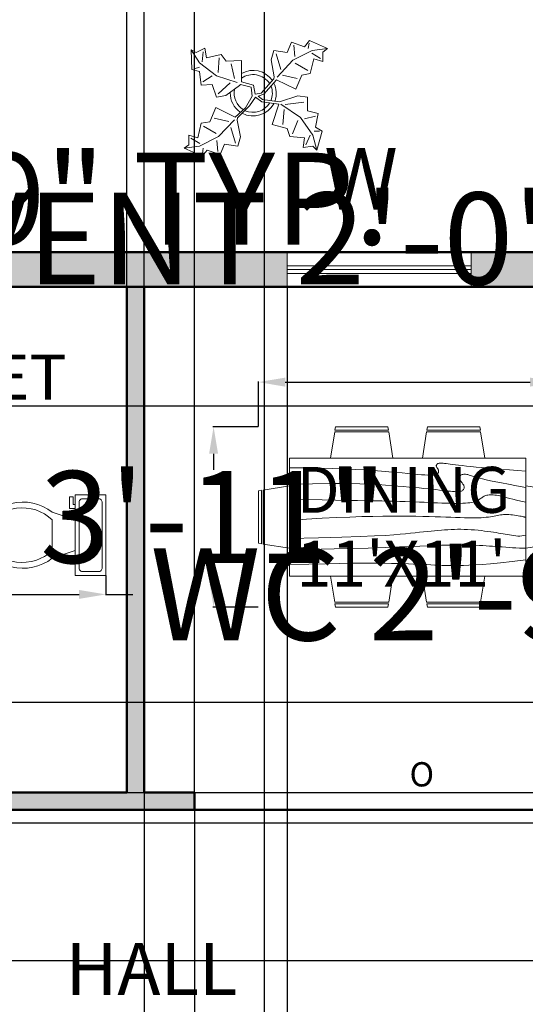
# Model space of a CAD drawing. Units: inches. Extents: x -166 to 1001, y 0 to 688.
# Tile 6 of 11: x 229 to 361, y 287 to 544. Entities that reach past the tile are written whole.
import ezdxf

# ---------------------------------------------------------------- set-up
doc = ezdxf.new("R2010")
doc.units = ezdxf.units.IN
doc.header["$MEASUREMENT"] = 0
for name, color, linetype, lineweight in [('A-ANNO-DIMS', 1, 'Continuous', 18), ('A-ANNO-TEXT', 2, 'Continuous', 25), ('A-AREA-IDEN', 2, 'Continuous', 25), ('A-FLOR-FIXT', 11, 'Continuous', 18), ('A-GLAZ', 130, 'Continuous', 18), ('A-WALL-PATT', 5, 'Continuous', 13), ('FURNITURE', 11, 'Continuous', 18), ('TREES', 80, 'Continuous', 13), ('WALLS', 250, 'Continuous', 50)]:
    doc.layers.add(name, color=color, linetype=linetype, lineweight=lineweight)
doc.styles.get("Standard").update_dxf_attribs({"font": 'arial.ttf'})
doc.dimstyles.get("Standard").update_dxf_attribs({"dimtxt": 24, "dimasz": 7, "dimexe": 0.18, "dimexo": 0.0625, "dimgap": 0.09, "dimtad": 0, "dimtih": 1, "dimtoh": 1, "dimdec": 0, "dimzin": 0, "dimdsep": 46, "dimlunit": 3, "dimtxsty": 'Standard', "dimcen": 0.09, "dimadec": 0, "dimazin": 0, "dimtfac": 1, "dimtdec": 0, "dimtofl": 0, "dimtmove": 0, "dimatfit": 3, "dimfxl": 1, "dimtolj": 1, "dimtzin": 0, "dimarcsym": 0})

# ---------------------------------------------------------------- blocks, each defined once
blk = doc.blocks.new('Toilet - top')
for p, q in [((9.5, -6), (9.5, -2)), ((-10, -8.5), (-8, -8.5)), ((-10, -9.5), (-10, -8.5)), ((-7, -9.5), (-10, -9.5)), ((-8, -8.5), (-8, -8)), ((-7, -8), (-7, -9.5)), ((-4, -8), (-6, -14)), ((4, -8), (6, -14)), ((4, -14), (-4, -14))]:
    blk.add_line(p, q)
blk.add_lwpolyline([(10.5, -8), (10.5, 0), (-10.5, 0), (-10.5, -8)], close=True)
for points in [[(-9.5, -2), (-9.5, -6)], [(8.5, -1), (-8.5, -1)], [(-8.5, -7), (8.5, -7)]]:
    blk.add_lwpolyline(points)
for centre, radius, start, end in [((-8.62, -1.88), 0.884, 81.8699, 188.1301), ((8.62, -1.88), 0.884, 351.8699, 98.1301), ((-8.62, -6.12), 0.884, 171.8699, 278.1301), ((8.62, -6.12), 0.884, 261.8699, 8.1301), ((3.52, -21.58), 12.17, 141.4691, 247.9714), ((4.2, -21.82), 11.33, 136.3677, 238.9468), ((-3.52, -21.58), 12.17, 292.0284, 38.5307), ((-4.2, -21.82), 11.33, 301.053, 43.6321), ((0, -27.88), 4, 245.7318, 294.2682), ((0, -29), 4, 254.8605, 285.1395)]:
    blk.add_arc(centre, radius, start, end)
blk = doc.blocks.new('Dining Set - 36 x 72 in.')
for p, q in [((-22, 27.5), (-22.1562, 26.50042)), ((-22, 27.5), (-6, 27.5)), ((-5.8437, 26.49966), (-6, 27.5)), ((6, 27.5), (5.8438, 26.50042)), ((6, 27.5), (22, 27.5)), ((22.1563, 26.49966), (22, 27.5)), ((-22.2343, 26.00059), (-23.4847, 17.99762)), ((-22.2304, 26), (-5.7608, 26)), ((-5.8416, 26.5), (-22.1534, 26.5)), ((-4.5152, 17.99762), (-5.7655, 25.99926)), ((5.7657, 26.00059), (4.5153, 17.99762)), ((5.7696, 26), (22.2392, 26)), ((22.1584, 26.5), (5.8466, 26.5)), ((23.4848, 17.99762), (22.2345, 25.99926)), ((36, 18), (-36, 18)), ((-36, 18), (-36, -18)), ((36, -18), (36, 18)), ((-44.0006, 8.23428), (-35.9976, 9.48474)), ((44.0006, 8.23428), (35.9976, 9.48474)), ((-45.5, 8), (-44.5004, 8.15617)), ((-45.5, 8), (-45.5, -8)), ((-44.5, -8.15843), (-44.5, 8.15338)), ((-44, 8.23041), (-44, -8.23915)), ((44, 8.23041), (44, -8.23915)), ((44.5, -8.15843), (44.5, 8.15338)), ((45.5, 8), (44.5005, 8.15617)), ((45.5, 8), (45.5, -8)), ((-44.4997, -8.15631), (-45.5, -8)), ((-35.9976, -9.48476), (-43.9993, -8.2345)), ((35.9976, -9.48476), (43.9993, -8.2345)), ((44.4997, -8.15631), (45.5, -8)), ((-36, -18), (36, -18)), ((-22.2343, -26.0006), (-23.4847, -17.99762)), ((-4.5152, -17.99762), (-5.7655, -25.99928)), ((5.7657, -26.0006), (4.5153, -17.99762)), ((23.4848, -17.99762), (22.2345, -25.99928)), ((-22.2304, -26), (-5.7608, -26)), ((-22, -27.5), (-22.1562, -26.50044)), ((-5.8416, -26.5), (-22.1534, -26.5)), ((-5.8437, -26.49967), (-6, -27.5)), ((5.7696, -26), (22.2392, -26)), ((6, -27.5), (5.8438, -26.50044)), ((22.1584, -26.5), (5.8466, -26.5)), ((22.1563, -26.49967), (22, -27.5)), ((-22, -27.5), (-6, -27.5)), ((6, -27.5), (22, -27.5))]:
    blk.add_line(p, q)
for points in [[(-36, 15), (-31.1772, 14.97754), (-26.8079, 14.91406), (-22.8538, 14.81543), (-19.276, 14.6875), (-16.0362, 14.53613), (-13.0957, 14.36718), (-10.4159, 14.18652), (-7.9583, 14), (-5.6904, 13.81315), (-3.6035, 13.63021), (-1.6954, 13.45508), (0.0365, 13.29166), (1.5945, 13.14388), (2.9811, 13.01562), (4.1988, 12.9108), (5.25, 12.83333), (6.1393, 12.78613), (6.8802, 12.76823), (7.4883, 12.77767), (7.9792, 12.8125), (8.3685, 12.87077), (8.6719, 12.95052), (8.9049, 13.0498), (9.0833, 13.16666), (9.2205, 13.29899), (9.3216, 13.44401), (9.3895, 13.59879), (9.4271, 13.76041), (9.4373, 13.92594), (9.4232, 14.09245), (9.3875, 14.257), (9.3333, 14.41666), (9.2638, 14.56917), (9.1836, 14.71484), (9.0975, 14.85465), (9.0104, 14.98958), (8.9272, 15.1206), (8.8529, 15.2487), (8.7922, 15.37483), (8.75, 15.5), (8.7305, 15.62467), (8.7344, 15.74739), (8.7617, 15.86621), (8.8125, 15.97916), (8.8867, 16.08431), (8.9844, 16.17968), (9.1055, 16.26334), (9.25, 16.33333), (9.4189, 16.38802), (9.6172, 16.42708), (9.8506, 16.45052), (10.125, 16.45833), (10.4463, 16.45052), (10.8203, 16.42708), (11.2529, 16.38802), (11.75, 16.33333), (12.3184, 16.26318), (12.9694, 16.17838), (13.7151, 16.07991), (14.5677, 15.96875), (15.5395, 15.84586), (16.6426, 15.71224), (17.8893, 15.56884), (19.2917, 15.41666), (20.859, 15.25667), (22.5879, 15.08984), (24.4721, 14.91715), (26.5052, 14.73958), (28.6809, 14.5581), (30.9929, 14.3737), (33.4347, 14.18733), (36, 14)], [(-36, 10), (-28.9766, 10.14274), (-23.1725, 10.20442), (-18.4241, 10.19775), (-14.5677, 10.13541), (-11.4399, 10.03011), (-8.877, 9.89453), (-6.7154, 9.74137), (-4.7917, 9.58333), (-2.9698, 9.43082), (-1.2246, 9.28515), (0.4415, 9.14534), (2.026, 9.01041), (3.5266, 8.87939), (4.9408, 8.7513), (6.266, 8.62516), (7.5, 8.5), (8.6411, 8.37549), (9.6914, 8.2539), (10.6538, 8.13818), (11.5312, 8.03125), (12.3267, 7.93603), (13.043, 7.85547), (13.6831, 7.79248), (14.25, 7.75), (14.7471, 7.7303), (15.1797, 7.73307), (15.5537, 7.75732), (15.875, 7.80208), (16.1494, 7.86637), (16.3828, 7.94922), (16.5811, 8.04964), (16.75, 8.16666), (16.8944, 8.29915), (17.0143, 8.44531), (17.1089, 8.60319), (17.1771, 8.77083), (17.218, 8.94629), (17.2305, 9.1276), (17.2137, 9.31282), (17.1667, 9.5), (17.0895, 9.6875), (16.987, 9.875), (16.8649, 10.0625), (16.7292, 10.25), (16.5856, 10.4375), (16.4401, 10.625), (16.2985, 10.8125), (16.1667, 11), (16.05, 11.18733), (15.9518, 11.3737), (15.8752, 11.5581), (15.8229, 11.73958), (15.798, 11.91715), (15.8034, 12.08984), (15.842, 12.25667), (15.9167, 12.41666), (16.0295, 12.56836), (16.1784, 12.70833), (16.3605, 12.83268), (16.5729, 12.9375), (16.8127, 13.01888), (17.0768, 13.07291), (17.3625, 13.0957), (17.6667, 13.08333), (17.9894, 13.03312), (18.3418, 12.94726), (18.7382, 12.82918), (19.1927, 12.68229), (19.7195, 12.51001), (20.3327, 12.31575), (21.0465, 12.10294), (21.875, 11.875), (22.8357, 11.63354), (23.959, 11.37304), (25.2786, 11.08618), (26.8282, 10.76562), (28.6414, 10.40405), (30.752, 9.99414), (33.1936, 9.52856), (36, 9)], [(-36, 5.5), (-30.7157, 5.3348), (-26.069, 5.20963), (-21.9946, 5.11767), (-18.4271, 5.05208), (-15.3009, 5.00602), (-12.5508, 4.97265), (-10.1112, 4.94515), (-7.9167, 4.91666), (-5.909, 4.88167), (-4.0586, 4.83984), (-2.3429, 4.79215), (-0.7396, 4.73958), (0.7739, 4.6831), (2.22, 4.6237), (3.6213, 4.56233), (5, 4.5), (6.373, 4.43782), (7.7344, 4.3776), (9.0723, 4.32129), (10.375, 4.27083), (11.6309, 4.22819), (12.8281, 4.19531), (13.9551, 4.17415), (15, 4.16666), (15.954, 4.17448), (16.819, 4.19791), (17.6001, 4.23698), (18.3021, 4.29166), (18.9299, 4.36198), (19.4883, 4.44791), (19.9823, 4.54948), (20.4167, 4.66666), (20.7969, 4.79899), (21.1302, 4.94401), (21.4245, 5.09879), (21.6875, 5.26041), (21.9271, 5.42594), (22.1511, 5.59245), (22.3672, 5.757), (22.5834, 5.91666), (22.8065, 6.06868), (23.0404, 6.21093), (23.2879, 6.34147), (23.5521, 6.45833), (23.8358, 6.55957), (24.142, 6.64323), (24.4735, 6.70735), (24.8334, 6.75), (25.2235, 6.76969), (25.642, 6.76692), (26.0858, 6.74267), (26.5521, 6.69791), (27.0379, 6.63362), (27.5404, 6.55078), (28.0565, 6.45036), (28.5834, 6.33333), (29.1242, 6.19987), (29.7071, 6.04687), (30.3661, 5.87044), (31.1354, 5.66666), (32.0493, 5.43164), (33.142, 5.16146), (34.4475, 4.85221), (36, 4.5)], [(-36, -1), (-30.7915, -0.6591), (-26.0195, -0.38216), (-21.6519, -0.16284), (-17.6563, 0.00521), (-14.0005, 0.12833), (-10.6523, 0.21289), (-7.5796, 0.26522), (-4.75, 0.29166), (-2.134, 0.29793), (0.2878, 0.28711), (2.5317, 0.26163), (4.6146, 0.22396), (6.5529, 0.17651), (8.3633, 0.12174), (10.0623, 0.06209), (11.6667, 0), (13.1899, -0.06201), (14.6341, -0.1211), (15.9982, -0.17432), (17.2813, -0.21875), (18.4823, -0.25147), (19.6003, -0.26953), (20.6343, -0.27002), (21.5834, -0.25), (22.4481, -0.20768), (23.2357, -0.14584), (23.9549, -0.06836), (24.6146, 0.02083), (25.2235, 0.11784), (25.7904, 0.21875), (26.3241, 0.31966), (26.8334, 0.41666), (27.3265, 0.50618), (27.8099, 0.58593), (28.2894, 0.65397), (28.7709, 0.70833), (29.2601, 0.74707), (29.763, 0.76823), (30.2855, 0.76985), (30.8334, 0.75), (31.4088, 0.70784), (31.9994, 0.64713), (32.589, 0.57275), (33.1615, 0.48958), (33.7008, 0.4025), (34.1908, 0.3164), (34.6153, 0.23616), (34.9584, 0.16666), (35.2099, 0.11165), (35.3848, 0.07031), (35.504, 0.04069), (35.5886, 0.02083), (35.6594, 0.00879), (35.7377, 0.0026), (35.8442, 0.00032), (36, 0)], [(-36, -6.5), (-27.1843, -6.31267), (-20.084, -6.1263), (-14.469, -5.9419), (-10.1094, -5.76042), (-6.7752, -5.58285), (-4.2363, -5.41016), (-2.2629, -5.24333), (-0.625, -5.08334), (0.8708, -4.93099), (2.2715, -4.78646), (3.5872, -4.64974), (4.8281, -4.52084), (6.0046, -4.39974), (7.127, -4.28646), (8.2053, -4.18099), (9.25, -4.08334), (10.2705, -3.99382), (11.2734, -3.91407), (12.2647, -3.84603), (13.25, -3.79167), (14.2354, -3.75293), (15.2266, -3.73177), (16.2295, -3.73015), (17.25, -3.75), (18.2912, -3.79248), (19.3451, -3.85547), (20.4009, -3.93604), (21.4479, -4.03125), (22.4754, -4.13819), (23.4727, -4.25391), (24.4289, -4.37549), (25.3334, -4.5), (26.1785, -4.62492), (26.9694, -4.74935), (27.7145, -4.87281), (28.4219, -4.99479), (29.1, -5.11483), (29.7572, -5.23242), (30.4016, -5.34709), (31.0417, -5.45834), (31.6837, -5.56437), (32.3262, -5.65821), (32.9658, -5.73153), (33.599, -5.77604), (34.2224, -5.78345), (34.8327, -5.74545), (35.4264, -5.65373), (36, -5.5)], [(-36, -10), (-26.4022, -9.81299), (-18.4675, -9.62891), (-11.9839, -9.45069), (-6.7396, -9.28125), (-2.5226, -9.12354), (0.8789, -8.98047), (3.6769, -8.85498), (6.0833, -8.75), (8.2767, -8.66765), (10.3021, -8.60677), (12.1712, -8.56543), (13.8958, -8.54167), (15.4876, -8.53353), (16.9583, -8.53907), (18.3197, -8.55632), (19.5834, -8.58334), (20.7616, -8.61841), (21.8685, -8.66081), (22.9188, -8.71004), (23.9271, -8.76563), (24.9081, -8.82707), (25.8763, -8.89388), (26.8465, -8.96558), (27.8334, -9.04167), (28.8474, -9.12118), (29.8828, -9.20117), (30.93, -9.27824), (31.9792, -9.34896), (33.0205, -9.40991), (34.0443, -9.45768), (35.0407, -9.48885), (36, -9.5)], [(-36, -14.5), (-30.0881, -14.33513), (-25.0332, -14.21224), (-20.7312, -14.12647), (-17.0781, -14.07292), (-13.97, -14.04671), (-11.3027, -14.04297), (-8.9724, -14.05681), (-6.875, -14.08334), (-4.9224, -14.11833), (-3.0905, -14.16016), (-1.3709, -14.20785), (0.2448, -14.26042), (1.7647, -14.3169), (3.1973, -14.3763), (4.5507, -14.43767), (5.8333, -14.5), (7.0554, -14.5621), (8.235, -14.62175), (9.3922, -14.67652), (10.5469, -14.72396), (11.7192, -14.76164), (12.929, -14.78711), (14.1965, -14.79794), (15.5417, -14.79167), (16.9933, -14.76424), (18.6152, -14.70508), (20.4804, -14.60197), (22.6615, -14.44271), (25.2312, -14.21509), (28.2624, -13.9069), (31.8277, -13.50594), (36, -13)]]:
    blk.add_lwpolyline(points)
blk = doc.blocks.new('Plant - Rubber or Philodendron')
for p, q in [((8.8871, 10.7908), (9.9809, 13.4933)), ((9.9809, 13.4933), (13.3837, 12.301)), ((13.3837, 12.301), (14.68, 13.9039)), ((14.5816, 13.2037), (14.3848, 11.8033)), ((14.68, 13.9039), (19.3848, 11.8146)), ((-16.2005, 11.4774), (-13.9899, 8.1064)), ((-16.2005, 11.4774), (-14.8639, 10.7964)), ((-16.0159, 6.3329), (-16.2005, 11.4774)), ((-14.8639, 10.7964), (-12.6195, 11.8975)), ((-13.3174, 8.325), (-13.0735, 11.0065)), ((-12.6195, 11.8975), (-12.1909, 9.4345)), ((-12.1909, 9.4345), (-8.3829, 10.3)), ((-8.3829, 10.3), (-7.0549, 8.501)), ((4.6914, 8.8812), (5.3859, 11.2828)), ((5.3859, 11.2828), (8.8871, 10.7908)), ((5.9878, 10.4842), (7.1971, 6.3869)), ((15.3859, 11.3055), (10.3916, 8.7942)), ((10.5828, 12.6946), (10.8893, 9.7953)), ((15.2875, 10.6053), (17.5907, 9.2105)), ((19.3848, 11.8146), (15.3859, 11.3055)), ((19.3848, 11.8146), (18.1868, 10.9119)), ((18.1868, 10.9119), (18.1925, 8.4119)), ((-13.9899, 8.1064), (-9.5434, 4.7185)), ((-8.8369, 9.409), (-9.0894, 5.6095)), ((-7.0549, 8.501), (-3.0284, 8.6941)), ((-4.8529, 4.012), (-5.7184, 7.82)), ((-3.0284, 8.6941), (-3.0709, 3.1041)), ((4.6914, 8.8812), (5.5014, 4.4831)), ((10.3916, 8.7942), (6.2847, 4.4028)), ((14.2977, 6.1031), (10.9934, 7.9956)), ((15.7909, 9.1065), (14.8995, 5.3044)), ((18.1925, 8.4119), (15.7909, 9.1065)), ((-14.0069, 5.8704), (-16.0159, 6.3329)), ((-15.3434, 6.5514), (-13.9984, 6.9884)), ((-13.5868, 2.2894), (-14.0069, 5.8704)), ((14.8995, 5.3044), (12.7005, 4.8994)), ((-13.1329, 3.1804), (-10.6614, 4.727)), ((-9.5434, 4.7185), (-4.1917, 2.9888)), ((-9.1318, 0.0195), (-5.9793, 2.9025)), ((-3.0709, 3.1041), (0.0797, 2.3163)), ((2.1141, 0.2298), (5.4346, 3.9146)), ((6.1032, 3.6844), (2.8262, -0.031)), ((5.4346, 3.9146), (5.5014, 4.4831)), ((11.1089, 1.1958), (6.1032, 3.6844)), ((7.7005, 4.8881), (11.5025, 3.9967)), ((12.7005, 4.8994), (11.1089, 1.1958)), ((-10.6784, 2.491), (-13.5868, 2.2894)), ((-9.5858, -0.8715), (-10.6784, 2.491)), ((-7.1228, -0.443), (-3.5248, 2.2131)), ((-3.5248, 2.2131), (-3.3011, 2.4355)), ((-3.3011, 2.4355), (-0.5306, 1.7947)), ((-0.5306, 1.7947), (-0.2255, -0.5527)), ((-0.5306, 1.7947), (-0.5306, 1.7947)), ((0.0797, 2.3163), (0.4866, -0.031)), ((0.4866, -0.031), (2.1141, 0.2298)), ((-7.1228, -0.443), (-9.5858, -0.8715)), ((-2.019, -3.6148), (-0.2255, -0.5527)), ((-0.9375, -3.1608), (0.5883, -0.8135)), ((0.5883, -0.8135), (2.2447, -2.0916)), ((2.8262, -0.031), (1.3003, -0.5527)), ((1.3003, -0.5527), (2.4193, -1.4655)), ((2.2447, -2.0916), (6.7108, -2.6626)), ((2.4193, -1.4655), (6.895, -2.1175)), ((11.6605, -0.5413), (6.895, -2.1175)), ((8.3544, -2.7453), (13.1973, -2.1704)), ((11.6605, -0.5413), (14.1354, -0.8948)), ((14.1354, -0.8948), (14.1354, -4.4304)), ((-11.3237, -7.2629), (-9.7321, -3.5593)), ((-9.7321, -3.5593), (-4.7264, -6.0479)), ((-2.019, -3.6148), (-4.7264, -6.0479)), ((-4.0579, -6.2781), (-0.9375, -3.1608)), ((4.943, -7.9659), (6.7108, -2.6626)), ((12.3677, -6.1981), (7.219, -2.6772)), ((8.125, -4.0768), (7.7715, -7.9659)), ((14.1354, -4.4304), (16.9638, -5.1375)), ((16.9638, -5.1375), (16.2567, -8.673)), ((-14.4141, -11.4699), (-13.5228, -7.6679)), ((-13.5228, -7.6679), (-11.3237, -7.2629)), ((-6.3237, -7.2516), (-10.1257, -6.3602)), ((-9.0148, -11.1577), (-4.9047, -6.8122)), ((-4.1246, -6.8466), (-4.0579, -6.2781)), ((-3.3146, -11.2447), (-4.1246, -6.8466)), ((10.2463, -10.4408), (11.6605, -6.9053)), ((15.5496, -10.7943), (12.3677, -6.1981)), ((16.2567, -5.8446), (13.4283, -6.5517)), ((-12.921, -8.4665), (-9.6166, -10.359)), ((-4.611, -12.8477), (-5.8203, -8.7504)), ((8.8321, -9.0266), (4.943, -7.9659)), ((9.5392, -11.1479), (8.8321, -9.0266)), ((17.3174, -9.7337), (15.9032, -9.7337)), ((16.2567, -8.673), (18.0245, -9.7337)), ((18.0245, -9.7337), (16.6103, -14.6834)), ((-16.8157, -10.7754), (-14.4141, -11.4699)), ((-16.8101, -13.2754), (-16.8157, -10.7754)), ((-13.9107, -12.9688), (-16.2139, -11.574)), ((-14.0091, -13.669), (-9.0148, -11.1577)), ((-9.206, -15.0581), (-9.5126, -12.1588)), ((-3.3146, -11.2447), (-4.0092, -13.6463)), ((13.4283, -11.5015), (9.5392, -11.1479)), ((13.0748, -13.9763), (13.4283, -11.5015)), ((14.8425, -10.7943), (13.7819, -13.2692)), ((16.6103, -14.6834), (15.5496, -10.7943)), ((-18.008, -14.1781), (-16.8101, -13.2754)), ((-18.008, -14.1781), (-14.0091, -13.669)), ((-13.3032, -16.2674), (-18.008, -14.1781)), ((-12.0069, -14.6645), (-13.3032, -16.2674)), ((-13.2048, -15.5672), (-13.008, -14.1668)), ((-8.6042, -15.8568), (-12.0069, -14.6645)), ((-7.5103, -13.1543), (-8.6042, -15.8568)), ((-4.0092, -13.6463), (-7.5103, -13.1543)), ((15.5496, -13.6228), (13.0748, -13.9763)), ((16.6103, -14.6834), (15.5496, -13.6228))]:
    blk.add_line(p, q)
for centre, radius, start, end in [((0, 0), 6.1275, 34.37569, 120.1028), ((-0.0601, -0.2075), 5.2461, 33.82192, 124.9414), ((-0.098, 0.1364), 6.1288, 341.2017, 26.09184), ((0.0308, 0.1664), 6, 178.6147, 235.1169), ((0.0308, 0.1664), 5, 168.1647, 238.6725), ((-0.2664, 0.1682), 5.2775, 338.4094, 20.03007), ((-0.1102, 0.4886), 5.2883, 247.3711, 327.472), ((-0.0234, 0.3825), 6.1492, 242.5812, 331.2714)]:
    blk.add_arc(centre, radius, start, end)
blk = doc.blocks.new('WIN-48IN')
for p, q in [((0, 4.5), (0, 9)), ((0, 9), (0, 0)), ((48, 9), (48, 0)), ((0, 5.5), (48, 5.5)), ((0, 4.5), (48, 4.5)), ((0, 3.5), (48, 3.5))]:
    blk.add_line(p, q)
blk = doc.blocks.new('*D19')
at = {"layer": 'A-ANNO-DIMS', "color": 0, "lineweight": -2, "transparency": 16777216}
for p, q in [((175.47, 483.8), (175.47, 487.52)), ((182.47, 487.34), (192.47, 487.34)), ((199.47, 483.8), (199.47, 487.52)), ((199.47, 487.34), (206.47, 487.34))]:
    blk.add_line(p, q, dxfattribs=at)
at = {"layer": 'A-ANNO-DIMS', "color": 0, "transparency": 16777216}
for points in [[(182.47, 488.51), (182.47, 486.17), (175.47, 487.34)], [(192.47, 488.51), (192.47, 486.17), (199.47, 487.34)]]:
    blk.add_solid(points, dxfattribs=at)
at = {"layer": 'Defpoints', "color": 0, "transparency": 16777216}
for p in [(199.47, 487.34), (175.47, 483.74), (199.47, 483.74)]:
    blk.add_point(p, dxfattribs=at)
at = {"layer": 'A-ANNO-DIMS', "color": 0, "transparency": 16777216, "insert": (329.7, 487.34), "char_height": 24, "attachment_point": 5}
blk.add_mtext('\\A1;VENT 2\'-0" TYP.', dxfattribs=at)
blk = doc.blocks.new('*D20')
at = {"layer": 'A-ANNO-DIMS', "color": 0, "lineweight": -2, "transparency": 16777216}
for p, q in [((171.87, 490.74), (171.87, 497.74)), ((171.87, 497.74), (178.87, 497.74)), ((175.41, 483.74), (171.69, 483.74)), ((175.41, 474.74), (171.69, 474.74)), ((171.87, 467.74), (171.87, 460.74))]:
    blk.add_line(p, q, dxfattribs=at)
at = {"layer": 'A-ANNO-DIMS', "color": 0, "transparency": 16777216}
for points in [[(170.71, 490.74), (173.04, 490.74), (171.87, 483.74)], [(170.71, 467.74), (173.04, 467.74), (171.87, 474.74)]]:
    blk.add_solid(points, dxfattribs=at)
at = {"layer": 'Defpoints', "color": 0, "transparency": 16777216}
for p in [(171.87, 483.74), (175.47, 483.74), (175.47, 474.74)]:
    blk.add_point(p, dxfattribs=at)
at = {"layer": 'A-ANNO-DIMS', "color": 0, "transparency": 16777216, "insert": (252.11, 497.74), "char_height": 24, "attachment_point": 5}
blk.add_mtext('\\A1;0\'-9" TYP.', dxfattribs=at)
blk = doc.blocks.new('*D25')
at = {"layer": 'A-ANNO-DIMS', "color": 0, "lineweight": -2, "transparency": 16777216}
for p, q in [((218.36, 399.34), (218.36, 394.26)), ((251.4, 399.34), (251.4, 394.26)), ((225.36, 394.44), (244.4, 394.44)), ((251.4, 394.44), (258.4, 394.44))]:
    blk.add_line(p, q, dxfattribs=at)
at = {"layer": 'A-ANNO-DIMS', "color": 0, "transparency": 16777216}
for points in [[(225.36, 395.61), (225.36, 393.27), (218.36, 394.44)], [(244.4, 395.61), (244.4, 393.27), (251.4, 394.44)]]:
    blk.add_solid(points, dxfattribs=at)
at = {"layer": 'Defpoints', "color": 0, "transparency": 16777216}
for p in [(218.36, 399.4), (251.4, 399.4), (251.4, 394.44)]:
    blk.add_point(p, dxfattribs=at)
at = {"layer": 'A-ANNO-DIMS', "color": 0, "transparency": 16777216, "insert": (364.72, 394.44), "char_height": 24, "attachment_point": 5}
blk.add_mtext('\\A1;WC 2\'-9" TYP.', dxfattribs=at)
blk = doc.blocks.new('*D33')
at = {"layer": 'A-ANNO-DIMS', "color": 0, "lineweight": -2, "transparency": 16777216}
for p, q in [((291.16, 438.23), (291.16, 450.03)), ((298.16, 449.85), (362.04, 449.85)), ((369.04, 438.23), (369.04, 450.03)), ((369.04, 449.85), (376.04, 449.85))]:
    blk.add_line(p, q, dxfattribs=at)
at = {"layer": 'A-ANNO-DIMS', "color": 0, "transparency": 16777216}
for points in [[(298.16, 451.02), (298.16, 448.68), (291.16, 449.85)], [(362.04, 451.02), (362.04, 448.68), (369.04, 449.85)]]:
    blk.add_solid(points, dxfattribs=at)
at = {"layer": 'Defpoints', "color": 0, "transparency": 16777216}
for p in [(369.04, 449.85), (291.16, 438.17), (369.04, 438.17)]:
    blk.add_point(p, dxfattribs=at)
at = {"layer": 'A-ANNO-DIMS', "color": 0, "transparency": 16777216, "insert": (508.03, 449.85), "char_height": 24, "attachment_point": 5}
blk.add_mtext('\\A1;DINING SET 6\'-6"', dxfattribs=at)
blk = doc.blocks.new('*D34')
at = {"layer": 'A-ANNO-DIMS', "color": 0, "lineweight": -2, "transparency": 16777216}
for p, q in [((291.1, 438.17), (279.3, 438.17)), ((279.48, 431.17), (279.48, 426.99)), ((279.48, 398.1), (279.48, 402.28)), ((291.1, 391.1), (279.3, 391.1))]:
    blk.add_line(p, q, dxfattribs=at)
at = {"layer": 'A-ANNO-DIMS', "color": 0, "transparency": 16777216}
for points in [[(278.31, 431.17), (280.65, 431.17), (279.48, 438.17)], [(278.31, 398.1), (280.65, 398.1), (279.48, 391.1)]]:
    blk.add_solid(points, dxfattribs=at)
at = {"layer": 'Defpoints', "color": 0, "transparency": 16777216}
for p in [(279.48, 438.17), (291.16, 438.17), (291.16, 391.1)]:
    blk.add_point(p, dxfattribs=at)
at = {"layer": 'A-ANNO-DIMS', "color": 0, "transparency": 16777216, "insert": (279.48, 414.63), "char_height": 24, "attachment_point": 5}
blk.add_mtext('\\A1;3\'-11"', dxfattribs=at)
blk = doc.blocks.new('*D35')
at = {"layer": 'A-ANNO-DIMS', "color": 0, "lineweight": -2, "transparency": 16777216}
for p, q in [((15.38, 483.8), (15.38, 593.07)), ((22.38, 592.89), (207.38, 592.89)), ((531.88, 592.89), (346.89, 592.89)), ((538.88, 483.8), (538.88, 593.07))]:
    blk.add_line(p, q, dxfattribs=at)
at = {"layer": 'A-ANNO-DIMS', "color": 0, "transparency": 16777216}
for points in [[(22.38, 594.06), (22.38, 591.72), (15.38, 592.89)], [(531.88, 594.06), (531.88, 591.72), (538.88, 592.89)]]:
    blk.add_solid(points, dxfattribs=at)
at = {"layer": 'Defpoints', "color": 0, "transparency": 16777216}
for p in [(538.88, 592.89), (15.38, 483.74), (538.88, 483.74)]:
    blk.add_point(p, dxfattribs=at)
at = {"layer": 'A-ANNO-DIMS', "color": 0, "transparency": 16777216, "insert": (277.13, 592.89), "char_height": 24, "attachment_point": 5}
blk.add_mtext('\\A1;43\'-7 1/2"', dxfattribs=at)
blk = doc.blocks.new('*D43')
at = {"layer": 'A-ANNO-DIMS', "color": 0, "lineweight": -2, "transparency": 16777216}
for p, q in [((160.88, 257.49), (160.88, 593.07)), ((167.88, 592.89), (201.62, 592.89)), ((208.62, 257.49), (208.62, 593.07)), ((208.62, 592.89), (215.62, 592.89))]:
    blk.add_line(p, q, dxfattribs=at)
at = {"layer": 'A-ANNO-DIMS', "color": 0, "transparency": 16777216}
for points in [[(167.88, 594.06), (167.88, 591.72), (160.88, 592.89)], [(201.62, 594.06), (201.62, 591.72), (208.62, 592.89)]]:
    blk.add_solid(points, dxfattribs=at)
at = {"layer": 'Defpoints', "color": 0, "transparency": 16777216}
for p in [(208.62, 592.89), (160.88, 257.42), (208.62, 257.42)]:
    blk.add_point(p, dxfattribs=at)
at = {"layer": 'A-ANNO-DIMS', "color": 0, "transparency": 16777216, "insert": (284.89, 592.89), "char_height": 24, "attachment_point": 5}
blk.add_mtext('\\A1;3\'-11 1/2"', dxfattribs=at)
blk = doc.blocks.new('*D44')
at = {"layer": 'A-ANNO-DIMS', "color": 0, "lineweight": -2, "transparency": 16777216}
for p, q in [((144.05, 474.68), (144.05, 35.41)), ((156.38, 474.68), (156.38, 35.41)), ((137.05, 35.59), (130.05, 35.59)), ((163.38, 35.59), (170.38, 35.59))]:
    blk.add_line(p, q, dxfattribs=at)
at = {"layer": 'A-ANNO-DIMS', "color": 0, "transparency": 16777216}
for points in [[(137.05, 36.76), (137.05, 34.42), (144.05, 35.59)], [(163.38, 36.76), (163.38, 34.42), (156.38, 35.59)]]:
    blk.add_solid(points, dxfattribs=at)
at = {"layer": 'Defpoints', "color": 0, "transparency": 16777216}
for p in [(144.05, 474.74), (156.38, 474.74), (156.38, 35.59)]:
    blk.add_point(p, dxfattribs=at)
at = {"layer": 'A-ANNO-DIMS', "color": 0, "transparency": 16777216, "insert": (229.2, 35.59), "char_height": 24, "attachment_point": 5}
blk.add_mtext('\\A1;1\'-0 1/2"', dxfattribs=at)
blk = doc.blocks.new('*D45')
at = {"layer": 'A-ANNO-DIMS', "color": 0, "lineweight": -2, "transparency": 16777216}
for p, q in [((160.88, 474.68), (160.88, 35.41)), ((175.47, 474.68), (175.47, 35.41)), ((167.88, 35.59), (168.47, 35.59)), ((175.47, 35.59), (182.47, 35.59))]:
    blk.add_line(p, q, dxfattribs=at)
at = {"layer": 'A-ANNO-DIMS', "color": 0, "transparency": 16777216}
for points in [[(167.88, 36.76), (167.88, 34.42), (160.88, 35.59)], [(168.47, 36.76), (168.47, 34.42), (175.47, 35.59)]]:
    blk.add_solid(points, dxfattribs=at)
at = {"layer": 'Defpoints', "color": 0, "transparency": 16777216}
for p in [(160.88, 474.74), (175.47, 474.74), (175.47, 35.59)]:
    blk.add_point(p, dxfattribs=at)
at = {"layer": 'A-ANNO-DIMS', "color": 0, "transparency": 16777216, "insert": (241.29, 35.59), "char_height": 24, "attachment_point": 5}
blk.add_mtext('\\A1;1\'-2 1/2"', dxfattribs=at)
blk = doc.blocks.new('*D46')
at = {"layer": 'A-ANNO-DIMS', "color": 0, "lineweight": -2, "transparency": 16777216}
for p, q in [((261.38, 474.68), (261.38, 35.41)), ((298.66, 474.68), (298.66, 35.41)), ((268.38, 35.59), (291.66, 35.59)), ((298.66, 35.59), (305.66, 35.59))]:
    blk.add_line(p, q, dxfattribs=at)
at = {"layer": 'A-ANNO-DIMS', "color": 0, "transparency": 16777216}
for points in [[(268.38, 36.76), (268.38, 34.42), (261.38, 35.59)], [(291.66, 36.76), (291.66, 34.42), (298.66, 35.59)]]:
    blk.add_solid(points, dxfattribs=at)
at = {"layer": 'Defpoints', "color": 0, "transparency": 16777216}
for p in [(261.38, 474.74), (298.66, 474.74), (298.66, 35.59)]:
    blk.add_point(p, dxfattribs=at)
at = {"layer": 'A-ANNO-DIMS', "color": 0, "transparency": 16777216, "insert": (365.61, 35.59), "char_height": 24, "attachment_point": 5}
blk.add_mtext('\\A1;3\'-1 1/2"', dxfattribs=at)
blk = doc.blocks.new('*D52')
at = {"layer": 'A-ANNO-DIMS', "color": 0, "lineweight": -2, "transparency": 16777216}
for p, q in [((675.03, 366.29), (675.03, 373.29)), ((675.03, 373.29), (682.03, 373.29)), ((24.44, 366.29), (675.21, 366.29)), ((675.03, 349.74), (675.03, 359.29)), ((24.44, 342.74), (675.21, 342.74))]:
    blk.add_line(p, q, dxfattribs=at)
at = {"layer": 'A-ANNO-DIMS', "color": 0, "transparency": 16777216}
for points in [[(673.87, 359.29), (676.2, 359.29), (675.03, 366.29)], [(673.87, 349.74), (676.2, 349.74), (675.03, 342.74)]]:
    blk.add_solid(points, dxfattribs=at)
at = {"layer": 'Defpoints', "color": 0, "transparency": 16777216}
for p in [(24.38, 366.29), (675.03, 366.29), (24.38, 342.74)]:
    blk.add_point(p, dxfattribs=at)
at = {"layer": 'A-ANNO-DIMS', "color": 0, "transparency": 16777216, "insert": (750.18, 373.29), "char_height": 24, "attachment_point": 5}
blk.add_mtext('\\A1;1\'-11 1/2"', dxfattribs=at)
blk = doc.blocks.new('*D55')
at = {"layer": 'A-ANNO-DIMS', "color": 0, "lineweight": -2, "transparency": 16777216}
for p, q in [((-120.77, 341.73), (-120.77, 348.73)), ((529.82, 334.73), (-120.95, 334.73)), ((529.82, 298.79), (-120.95, 298.79)), ((-120.77, 291.79), (-120.77, 284.79))]:
    blk.add_line(p, q, dxfattribs=at)
at = {"layer": 'A-ANNO-DIMS', "color": 0, "transparency": 16777216}
for points in [[(-121.93, 341.73), (-119.6, 341.73), (-120.77, 334.73)], [(-121.93, 291.79), (-119.6, 291.79), (-120.77, 298.79)]]:
    blk.add_solid(points, dxfattribs=at)
at = {"layer": 'Defpoints', "color": 0, "transparency": 16777216}
for p in [(-120.77, 334.73), (529.88, 334.73), (529.88, 298.79)]:
    blk.add_point(p, dxfattribs=at)
at = {"layer": 'A-ANNO-DIMS', "color": 0, "transparency": 16777216, "insert": (-120.77, 316.76), "char_height": 24, "attachment_point": 5}
blk.add_mtext('\\A1;3\'-0"', dxfattribs=at)
blk = doc.blocks.new('*D60')
at = {"layer": 'A-ANNO-DIMS', "color": 0, "lineweight": -2, "transparency": 16777216}
for p, q in [((156.38, 342.68), (156.38, 35.41)), ((146.03, 338.18), (146.03, 35.41)), ((139.03, 35.59), (132.03, 35.59)), ((163.38, 35.59), (170.38, 35.59))]:
    blk.add_line(p, q, dxfattribs=at)
at = {"layer": 'A-ANNO-DIMS', "color": 0, "transparency": 16777216}
for points in [[(139.03, 36.76), (139.03, 34.42), (146.03, 35.59)], [(163.38, 36.76), (163.38, 34.42), (156.38, 35.59)]]:
    blk.add_solid(points, dxfattribs=at)
at = {"layer": 'Defpoints', "color": 0, "transparency": 16777216}
for p in [(156.38, 342.74), (146.03, 338.24), (156.38, 35.59)]:
    blk.add_point(p, dxfattribs=at)
at = {"layer": 'A-ANNO-DIMS', "color": 0, "transparency": 16777216, "insert": (239.66, 35.59), "char_height": 24, "attachment_point": 5}
blk.add_mtext('\\A1;0\'-10 1/2"', dxfattribs=at)
blk = doc.blocks.new('*D61')
at = {"layer": 'A-ANNO-DIMS', "color": 0, "lineweight": -2, "transparency": 16777216}
for p, q in [((171.55, 342.8), (171.55, 593.07)), ((178.55, 592.89), (194.55, 592.89)), ((201.55, 342.8), (201.55, 593.07)), ((201.55, 592.89), (208.55, 592.89))]:
    blk.add_line(p, q, dxfattribs=at)
at = {"layer": 'A-ANNO-DIMS', "color": 0, "transparency": 16777216}
for points in [[(178.55, 594.06), (178.55, 591.72), (171.55, 592.89)], [(194.55, 594.06), (194.55, 591.72), (201.55, 592.89)]]:
    blk.add_solid(points, dxfattribs=at)
at = {"layer": 'Defpoints', "color": 0, "transparency": 16777216}
for p in [(201.55, 592.89), (171.55, 342.74), (201.55, 342.74)]:
    blk.add_point(p, dxfattribs=at)
at = {"layer": 'A-ANNO-DIMS', "color": 0, "transparency": 16777216, "insert": (240.75, 592.89), "char_height": 24, "attachment_point": 5}
blk.add_mtext('\\A1;2\'-6"', dxfattribs=at)
blk = doc.blocks.new('*D62')
at = {"layer": 'A-ANNO-DIMS', "color": 0, "lineweight": -2, "transparency": 16777216}
for p, q in [((201.55, 342.8), (201.55, 593.07)), ((208.55, 592.89), (249.88, 592.89)), ((256.88, 342.8), (256.88, 593.07)), ((256.88, 592.89), (263.88, 592.89))]:
    blk.add_line(p, q, dxfattribs=at)
at = {"layer": 'A-ANNO-DIMS', "color": 0, "transparency": 16777216}
for points in [[(208.55, 594.06), (208.55, 591.72), (201.55, 592.89)], [(249.88, 594.06), (249.88, 591.72), (256.88, 592.89)]]:
    blk.add_solid(points, dxfattribs=at)
at = {"layer": 'Defpoints', "color": 0, "transparency": 16777216}
for p in [(256.88, 592.89), (201.55, 342.74), (256.88, 342.74)]:
    blk.add_point(p, dxfattribs=at)
at = {"layer": 'A-ANNO-DIMS', "color": 0, "transparency": 16777216, "insert": (324.32, 592.89), "char_height": 24, "attachment_point": 5}
blk.add_mtext('\\A1;4\'-7 1/2"', dxfattribs=at)
blk = doc.blocks.new('*D63')
at = {"layer": 'A-ANNO-DIMS', "color": 0, "lineweight": -2, "transparency": 16777216}
for p, q in [((274.49, 338.18), (274.49, 35.41)), ((384.24, 338.18), (384.24, 35.41)), ((281.49, 35.59), (377.24, 35.59)), ((384.24, 35.59), (391.24, 35.59))]:
    blk.add_line(p, q, dxfattribs=at)
at = {"layer": 'A-ANNO-DIMS', "color": 0, "transparency": 16777216}
for points in [[(281.49, 36.76), (281.49, 34.42), (274.49, 35.59)], [(377.24, 36.76), (377.24, 34.42), (384.24, 35.59)]]:
    blk.add_solid(points, dxfattribs=at)
at = {"layer": 'Defpoints', "color": 0, "transparency": 16777216}
for p in [(274.49, 338.24), (384.24, 338.24), (384.24, 35.59)]:
    blk.add_point(p, dxfattribs=at)
at = {"layer": 'A-ANNO-DIMS', "color": 0, "transparency": 16777216, "insert": (451.19, 35.59), "char_height": 24, "attachment_point": 5}
blk.add_mtext('\\A1;9\'-1 1/2"', dxfattribs=at)
blk = doc.blocks.new('*D64')
at = {"layer": 'A-ANNO-DIMS', "color": 0, "lineweight": -2, "transparency": 16777216}
for p, q in [((254.38, 592.89), (247.38, 592.89)), ((261.38, 342.8), (261.38, 593.07)), ((274.49, 342.8), (274.49, 593.07)), ((281.49, 592.89), (288.49, 592.89))]:
    blk.add_line(p, q, dxfattribs=at)
at = {"layer": 'A-ANNO-DIMS', "color": 0, "transparency": 16777216}
for points in [[(254.38, 594.06), (254.38, 591.72), (261.38, 592.89)], [(281.49, 594.06), (281.49, 591.72), (274.49, 592.89)]]:
    blk.add_solid(points, dxfattribs=at)
at = {"layer": 'Defpoints', "color": 0, "transparency": 16777216}
for p in [(274.49, 592.89), (261.38, 342.74), (274.49, 342.74)]:
    blk.add_point(p, dxfattribs=at)
at = {"layer": 'A-ANNO-DIMS', "color": 0, "transparency": 16777216, "insert": (319.35, 592.89), "char_height": 24, "attachment_point": 5}
blk.add_mtext('\\A1;1\'-1"', dxfattribs=at)
blk = doc.blocks.new('*D75')
at = {"layer": 'A-ANNO-DIMS', "color": 0, "lineweight": -2, "transparency": 16777216}
for p, q in [((-120.77, 481.74), (-120.77, 488.74)), ((529.82, 474.74), (-120.95, 474.74)), ((529.82, 443.59), (-120.95, 443.59)), ((-120.77, 436.59), (-120.77, 429.59))]:
    blk.add_line(p, q, dxfattribs=at)
at = {"layer": 'A-ANNO-DIMS', "color": 0, "transparency": 16777216}
for points in [[(-121.93, 481.74), (-119.6, 481.74), (-120.77, 474.74)], [(-121.93, 436.59), (-119.6, 436.59), (-120.77, 443.59)]]:
    blk.add_solid(points, dxfattribs=at)
at = {"layer": 'Defpoints', "color": 0, "transparency": 16777216}
for p in [(529.88, 474.74), (-120.77, 443.59), (529.88, 443.59)]:
    blk.add_point(p, dxfattribs=at)
at = {"layer": 'A-ANNO-DIMS', "color": 0, "transparency": 16777216, "insert": (-120.77, 459.16), "char_height": 24, "attachment_point": 5}
blk.add_mtext('\\A1;2\'-7"', dxfattribs=at)
blk = doc.blocks.new('*D78')
at = {"layer": 'A-ANNO-DIMS', "color": 0, "lineweight": -2, "transparency": 16777216}
for p, q in [((160.88, 153.8), (160.88, 593.07)), ((167.88, 592.89), (186.64, 592.89)), ((285.77, 592.89), (267.01, 592.89)), ((292.77, 153.8), (292.77, 593.07))]:
    blk.add_line(p, q, dxfattribs=at)
at = {"layer": 'A-ANNO-DIMS', "color": 0, "transparency": 16777216}
for points in [[(167.88, 594.06), (167.88, 591.72), (160.88, 592.89)], [(285.77, 594.06), (285.77, 591.72), (292.77, 592.89)]]:
    blk.add_solid(points, dxfattribs=at)
at = {"layer": 'Defpoints', "color": 0, "transparency": 16777216}
for p in [(292.77, 592.89), (160.88, 153.74), (292.77, 153.74)]:
    blk.add_point(p, dxfattribs=at)
at = {"layer": 'A-ANNO-DIMS', "color": 0, "transparency": 16777216, "insert": (226.83, 592.89), "char_height": 24, "attachment_point": 5}
blk.add_mtext('\\A1;11\'-0"', dxfattribs=at)

msp = doc.modelspace()

# ---------------------------------------------------------------- hatches: boundary and pattern name
at = {"layer": 'A-WALL-PATT'}
h = msp.add_hatch(color=256, dxfattribs=at)
h.dxf.hatch_style = 1
h.paths.add_polyline_path([(96.05, 483.74), (15.38, 483.74), (15.38, 414.29), (24.38, 414.29), (24.38, 474.74), (96.05, 474.74)])
h.paths.add_polyline_path([(175.47, 483.74), (144.05, 483.74), (144.05, 474.74), (156.38, 474.74), (175.47, 474.74)])
h.paths.add_polyline_path([(298.66, 483.74), (199.47, 483.74), (199.47, 474.74), (256.88, 474.74), (298.66, 474.74)])
h.paths.add_polyline_path([(430.46, 483.74), (346.66, 483.74), (346.66, 474.74), (393.38, 474.74), (430.46, 474.74)])
h.paths.add_polyline_path([(261.38, 474.74), (256.88, 474.74), (256.88, 342.74), (201.55, 342.74), (201.55, 338.24), (274.49, 338.24), (274.49, 342.74), (261.38, 342.74)])
h.paths.add_polyline_path([(160.88, 474.74), (156.38, 474.74), (156.38, 342.74), (146.03, 342.74), (146.03, 338.24), (171.55, 338.24), (171.55, 342.74), (160.88, 342.74)])
h.paths.add_polyline_path([(397.88, 474.74), (393.38, 474.74), (393.38, 383.21), (397.88, 383.21)])
h.paths.add_polyline_path([(538.88, 362.18), (529.88, 362.18), (529.88, 342.74), (397.88, 342.74), (397.88, 348.69), (393.38, 348.69), (393.38, 342.74), (384.24, 342.74), (384.24, 338.24), (529.88, 338.24), (529.88, 334.73), (538.88, 334.73)])
h.paths.add_polyline_path([(538.88, 483.74), (478.46, 483.74), (478.46, 474.74), (529.88, 474.74), (529.88, 410.18), (538.88, 410.18)])
h.paths.add_polyline_path([(538.88, 298.79), (529.88, 298.79), (529.88, 278.24), (442.61, 278.24), (442.61, 273.74), (529.88, 273.74), (529.88, 221.94), (538.88, 221.94)])
h.paths.add_polyline_path([(538.88, 173.94), (529.88, 173.94), (529.88, 153.74), (393.38, 153.74), (382.23, 153.74), (382.23, 144.74), (538.88, 144.74)])
h.paths.add_polyline_path([(397.88, 164.32), (393.38, 164.32), (393.38, 153.74), (397.88, 153.74)], flags=17)
h.paths.add_polyline_path([(397.88, 273.74), (406.66, 273.74), (406.66, 278.24), (393.38, 278.24), (393.38, 273.74), (393.38, 230.24), (316.88, 230.24), (316.88, 153.74), (321.38, 153.74), (321.38, 225.74), (393.38, 225.74), (393.38, 194.32), (397.88, 194.32)])
h.paths.add_polyline_path([(358.23, 153.74), (316.88, 153.74), (284.58, 153.74), (284.58, 144.74), (358.23, 144.74)])
h.paths.add_polyline_path([(224.58, 153.74), (156.38, 153.74), (149.31, 153.74), (149.31, 144.74), (224.58, 144.74)])
h.paths.add_polyline_path([(101.31, 153.74), (24.38, 153.74), (24.38, 168.41), (15.38, 168.41), (15.38, 144.74), (101.31, 144.74)])
h.paths.add_polyline_path([(160.88, 273.74), (160.88, 278.24), (147.87, 278.24), (147.87, 273.74), (156.38, 273.74), (156.38, 153.74), (160.88, 153.74)])
h.paths.add_polyline_path([(111.92, 278.24), (100.88, 278.24), (100.88, 338.24), (110.03, 338.24), (110.03, 342.74), (24.38, 342.74), (24.38, 366.29), (15.38, 366.29), (15.38, 216.41), (24.38, 216.41), (24.38, 273.74), (44.93, 273.74), (44.93, 278.24), (24.38, 278.24), (24.38, 338.24), (96.38, 338.24), (96.38, 278.24), (74.93, 278.24), (74.93, 273.74), (111.92, 273.74)])

# ---------------------------------------------------------------- linework, layer by layer
at = {"layer": 'WALLS'}
for p, q in [((15.38, 483.74), (538.88, 483.74)), ((156.38, 474.74), (256.88, 474.74)), ((256.88, 342.74), (256.88, 474.74)), ((256.88, 474.74), (393.38, 474.74)), ((261.38, 342.74), (261.38, 474.74)), ((201.55, 342.74), (256.88, 342.74)), ((261.38, 342.74), (274.49, 342.74)), ((274.49, 342.74), (274.49, 338.24)), ((201.55, 338.24), (529.88, 338.24))]:
    msp.add_line(p, q, dxfattribs=at)

# ---------------------------------------------------------------- block references
at = {"layer": 'A-FLOR-FIXT', "rotation": 270}
msp.add_blockref('Toilet - top', (251.4, 409.9), dxfattribs=at)
at = {"layer": 'A-GLAZ'}
msp.add_blockref('WIN-48IN', (298.66, 474.74), dxfattribs=at)
at = {"layer": 'FURNITURE', "xscale": 0.8558305474851317, "yscale": 0.8558305474851317, "zscale": 0.8558305474851317}
msp.add_blockref('Dining Set - 36 x 72 in.', (330.1, 414.63), dxfattribs=at)
at = {"layer": 'TREES'}
msp.add_blockref('Plant - Rubber or Philodendron', (289.8, 525.09), dxfattribs=at)

# ---------------------------------------------------------------- texts
at = {"layer": 'A-ANNO-TEXT'}
msp.add_text('W ', height=16.096, dxfattribs=at).set_placement((308.3, 494.89))
msp.add_text('O', height=6.33, rotation=180, dxfattribs=at).set_placement((337, 350.65))
at = {"layer": 'A-AREA-IDEN'}
for s, height, p in [('C.TOILET', 11.769, (172.36, 445.27)), ('DINING', 11.989, (301.13, 415.74)), ("11'X11'", 11.989, (301.13, 396.48)), ('HALL', 13.567, (240.9, 289.91))]:
    msp.add_text(s, height=height, dxfattribs=at).set_placement(p)

# ---------------------------------------------------------------- dimensions: what is measured, and where the dimension line sits
at = {"layer": 'A-ANNO-DIMS'}
for base, p1, p2, picture, middle in [((538.88, 592.89), (15.38, 483.74), (538.88, 483.74), '*D35', (277.13, 592.89)), ((208.62, 592.89), (160.88, 257.42), (208.62, 257.42), '*D43', (284.89, 592.89)), ((256.88, 592.89), (201.55, 342.74), (256.88, 342.74), '*D62', (324.32, 592.89)), ((292.77, 592.89), (160.88, 153.74), (292.77, 153.74), '*D78', (226.83, 592.89)), ((201.55, 592.89), (171.55, 342.74), (201.55, 342.74), '*D61', (240.75, 592.89)), ((274.49, 592.89), (261.38, 342.74), (274.49, 342.74), '*D64', (319.35, 592.89)), ((156.38, 35.59), (144.05, 474.74), (156.38, 474.74), '*D44', (229.2, 35.59)), ((175.47, 35.59), (160.88, 474.74), (175.47, 474.74), '*D45', (241.29, 35.59)), ((298.66, 35.59), (261.38, 474.74), (298.66, 474.74), '*D46', (365.61, 35.59)), ((156.3825, 35.5909), (146.0262, 338.2409), (156.3825, 342.7409), '*D60', (239.6566, 35.5909)), ((384.2404, 35.5909), (274.4932, 338.2409), (384.2404, 338.2409), '*D63', (451.1912, 35.5909))]:
    dim = msp.add_linear_dim(base=base, p1=p1, p2=p2, dimstyle='Standard', override={"dimdec": 1, "dimlfac": 1, "dimrnd": 0, "dimzin": 1, "dimdsep": 46, "dimlunit": 4, "dimfrac": 2}, dxfattribs=at)
    dim.commit()
    dim.dimension.update_dxf_attribs({"geometry": picture, "text_midpoint": middle})
for base, p1, p2, text, picture, middle in [((199.47, 487.34), (175.47, 483.74), (199.47, 483.74), 'VENT <> TYP.', '*D19', (329.7, 487.34)), ((369.04, 449.85), (291.16, 438.17), (369.04, 438.17), 'DINING SET <>', '*D33', (508.03, 449.85)), ((251.4, 394.44), (218.36, 399.4), (251.4, 399.4), 'WC <> TYP.', '*D25', (364.72, 394.44))]:
    dim = msp.add_linear_dim(base=base, p1=p1, p2=p2, text=text, dimstyle='Standard', override={"dimdec": 1, "dimlfac": 1, "dimrnd": 0, "dimzin": 1, "dimdsep": 46, "dimlunit": 4, "dimfrac": 2}, dxfattribs=at)
    dim.commit()
    dim.dimension.update_dxf_attribs({"geometry": picture, "text_midpoint": middle})
dim = msp.add_linear_dim(base=(171.87, 483.74), p1=(175.47, 474.74), p2=(175.47, 483.74), angle=90, text='<> TYP.', dimstyle='Standard', override={"dimdec": 1, "dimlfac": 1, "dimrnd": 0, "dimzin": 1, "dimdsep": 46, "dimlunit": 4, "dimfrac": 2}, dxfattribs=at)
dim.commit()
dim.dimension.update_dxf_attribs({"geometry": '*D20', "text_midpoint": (252.11, 497.74)})
for base, p1, p2, picture, middle in [((-120.7675, 443.5862), (529.8825, 474.7409), (529.8825, 443.5862), '*D75', (-120.7675, 459.1635)), ((279.48, 438.17), (291.16, 391.1), (291.16, 438.17), '*D34', (279.48, 414.63)), ((675.0325, 366.2884), (24.3825, 342.7409), (24.3825, 366.2884), '*D52', (750.177, 373.2884)), ((-120.77, 334.73), (529.88, 298.79), (529.88, 334.73), '*D55', (-120.77, 316.76))]:
    dim = msp.add_linear_dim(base=base, p1=p1, p2=p2, angle=90, dimstyle='Standard', override={"dimdec": 1, "dimlfac": 1, "dimrnd": 0, "dimzin": 1, "dimdsep": 46, "dimlunit": 4, "dimfrac": 2}, dxfattribs=at)
    dim.commit()
    dim.dimension.update_dxf_attribs({"geometry": picture, "text_midpoint": middle})

doc.saveas('drawing.dxf')
